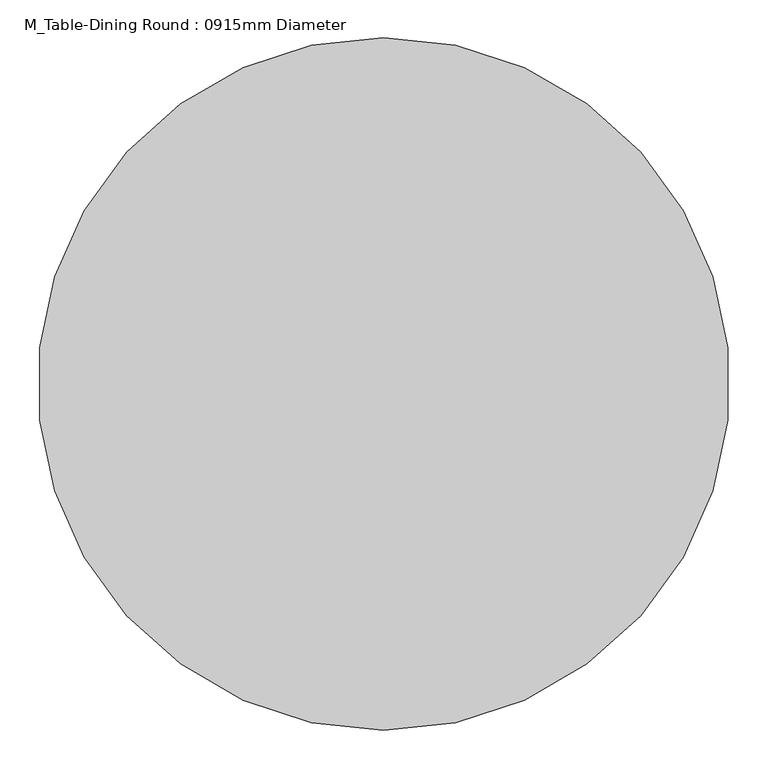
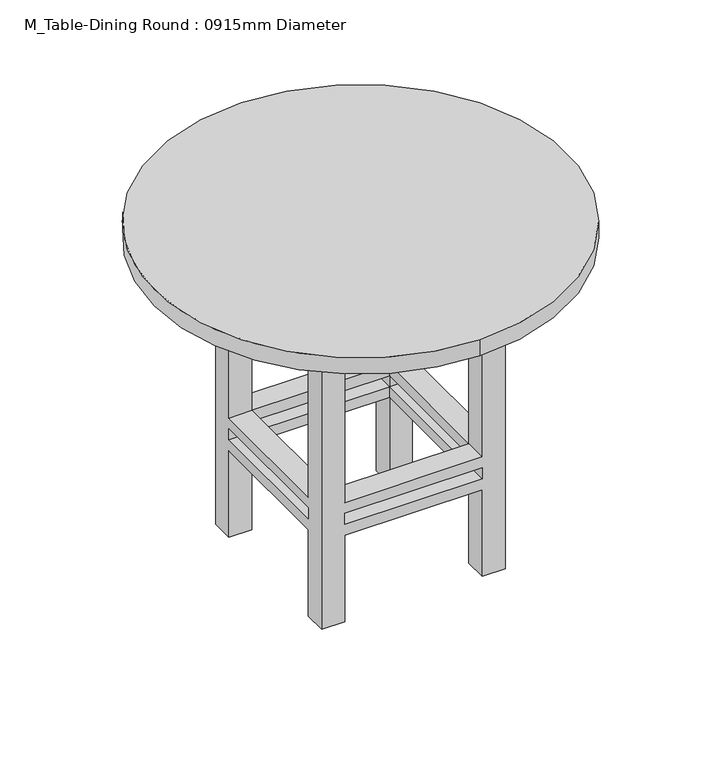
"""IFC4 building model written with IfcOpenShell, lengths in millimetres: furniture geometry, M_Table-Dining Round : 0915mm Diameter."""

from ifc_helpers import new_model, si_unit, point, frame, frame_2d, origin, place, context, project, spatial, polyline, circle_curve, trimmed, segment, composite_curve, outline, extrude, faceted_brep, source, transform, mapped, element, save


def m_table_dining_round_0915mm_diameter_394c0b6d(model_context):
    return source(origin(), model_context, "Body", "SolidModel", [
        extrude(outline(polyline([(332.4319672, 43.8713115), (332.4319672, -413.6286885), (-125.0680328, -413.6286885), (-125.0680328, 43.8713115), (332.4319672, 43.8713115)]), holes=[polyline([(307.0319672, 18.4713115), (-99.6680328, 18.4713115), (-99.6680328, -388.2286885), (307.0319672, -388.2286885), (307.0319672, 18.4713115)])]), frame((0.0, 0.0, 647.7), z_axis=(0.0, 0.0, 1.0), x_axis=(1.0, 0.0, 0.0)), (0.0, 0.0, 1.0), 76.2),
        faceted_brep([(-48.8680328, 18.4713115, 647.7), (-99.6680328, 18.4713115, 647.7), (-99.6680328, -32.3286885, 647.7), (-48.8680328, -32.3286885, 647.7), (256.2319672, 18.4713115, 647.7), (256.2319672, -32.3286885, 647.7), (307.0319672, -32.3286885, 647.7), (307.0319672, 18.4713115, 647.7), (256.2319672, -388.2286885, 647.7), (307.0319672, -388.2286885, 647.7), (307.0319672, -337.4286885, 647.7), (256.2319672, -337.4286885, 647.7), (-48.8680328, -388.2286885, 647.7), (-48.8680328, -337.4286885, 647.7), (-99.6680328, -337.4286885, 647.7), (-99.6680328, -388.2286885, 647.7), (-48.8680328, 18.4713115, 0.0), (-48.8680328, -32.3286885, 0.0), (-99.6680328, -32.3286885, 0.0), (-99.6680328, 18.4713115, 0.0), (256.2319672, 18.4713115, 0.0), (307.0319672, 18.4713115, 0.0), (307.0319672, -32.3286885, 0.0), (256.2319672, -32.3286885, 0.0), (256.2319672, -388.2286885, 0.0), (256.2319672, -337.4286885, 0.0), (307.0319672, -337.4286885, 0.0), (307.0319672, -388.2286885, 0.0), (-48.8680328, -388.2286885, 0.0), (-99.6680328, -388.2286885, 0.0), (-99.6680328, -337.4286885, 0.0), (-48.8680328, -337.4286885, 0.0), (-48.8680328, 18.4713115, 279.4), (256.2319672, 18.4713115, 279.4), (256.2319672, 18.4713115, 203.2), (-48.8680328, 18.4713115, 203.2), (256.2319672, 18.4713115, 228.6), (256.2319672, 18.4713115, 254.0), (-48.8680328, 18.4713115, 254.0), (-48.8680328, 18.4713115, 228.6), (-99.6680328, -32.3286885, 203.2), (-99.6680328, -337.4286885, 203.2), (-99.6680328, -337.4286885, 279.4), (-99.6680328, -32.3286885, 279.4), (-99.6680328, -32.3286885, 228.6), (-99.6680328, -32.3286885, 254.0), (-99.6680328, -337.4286885, 254.0), (-99.6680328, -337.4286885, 228.6), (-48.8680328, -32.3286885, 279.4), (-48.8680328, -32.3286885, 203.2), (-48.8680328, -32.3286885, 228.6), (-48.8680328, -32.3286885, 254.0), (256.2319672, -32.3286885, 279.4), (256.2319672, -32.3286885, 203.2), (256.2319672, -32.3286885, 228.6), (256.2319672, -32.3286885, 254.0), (307.0319672, -32.3286885, 279.4), (307.0319672, -32.3286885, 203.2), (307.0319672, -32.3286885, 228.6), (307.0319672, -32.3286885, 254.0), (307.0319672, -337.4286885, 279.4), (307.0319672, -337.4286885, 203.2), (307.0319672, -337.4286885, 228.6), (307.0319672, -337.4286885, 254.0), (256.2319672, -388.2286885, 279.4), (-48.8680328, -388.2286885, 279.4), (-48.8680328, -388.2286885, 203.2), (256.2319672, -388.2286885, 203.2), (-48.8680328, -388.2286885, 228.6), (-48.8680328, -388.2286885, 254.0), (256.2319672, -388.2286885, 254.0), (256.2319672, -388.2286885, 228.6), (256.2319672, -337.4286885, 279.4), (256.2319672, -337.4286885, 203.2), (256.2319672, -337.4286885, 228.6), (256.2319672, -337.4286885, 254.0), (-48.8680328, -337.4286885, 279.4), (-48.8680328, -337.4286885, 203.2), (-48.8680328, -337.4286885, 228.6), (-48.8680328, -337.4286885, 254.0)], [[[0, 1, 2, 3]], [[4, 5, 6, 7]], [[8, 9, 10, 11]], [[12, 13, 14, 15]], [[16, 17, 18, 19]], [[20, 21, 22, 23]], [[24, 25, 26, 27]], [[28, 29, 30, 31]], [[1, 0, 32, 33, 4, 7, 21, 20, 34, 35, 16, 19], [36, 37, 38, 39]], [[2, 1, 19, 18, 40, 41, 30, 29, 15, 14, 42, 43], [44, 45, 46, 47]], [[3, 2, 43, 48]], [[18, 17, 49, 40]], [[44, 50, 51, 45]], [[0, 3, 48, 32]], [[17, 16, 35, 49]], [[50, 39, 38, 51]], [[5, 4, 33, 52]], [[20, 23, 53, 34]], [[36, 54, 55, 37]], [[6, 5, 52, 56]], [[23, 22, 57, 53]], [[54, 58, 59, 55]], [[21, 7, 6, 56, 60, 10, 9, 27, 26, 61, 57, 22], [62, 63, 59, 58]], [[27, 9, 8, 64, 65, 12, 15, 29, 28, 66, 67, 24], [68, 69, 70, 71]], [[11, 10, 60, 72]], [[26, 25, 73, 61]], [[62, 74, 75, 63]], [[8, 11, 72, 64]], [[25, 24, 67, 73]], [[74, 71, 70, 75]], [[13, 12, 65, 76]], [[28, 31, 77, 66]], [[68, 78, 79, 69]], [[14, 13, 76, 42]], [[31, 30, 41, 77]], [[78, 47, 46, 79]], [[54, 74, 62, 58]], [[74, 78, 68, 71]], [[78, 50, 44, 47]], [[50, 54, 36, 39]], [[53, 49, 35, 34]], [[49, 77, 41, 40]], [[77, 73, 67, 66]], [[73, 53, 57, 61]], [[74, 54, 53, 73]], [[78, 74, 73, 77]], [[50, 78, 77, 49]], [[54, 50, 49, 53]], [[52, 72, 60, 56]], [[72, 76, 65, 64]], [[76, 48, 43, 42]], [[48, 52, 33, 32]], [[55, 51, 38, 37]], [[51, 79, 46, 45]], [[79, 75, 70, 69]], [[75, 55, 59, 63]], [[72, 52, 55, 75]], [[76, 72, 75, 79]], [[48, 76, 79, 51]], [[52, 48, 51, 55]]]),
        extrude(outline(composite_curve([segment(trimmed(circle_curve(frame_2d((103.6819672, -184.8786885)), 457.5), [point((103.6819672, -642.3786885))], [point((103.6819672, 272.6213115))], False, "CARTESIAN"), True, "CONTINUOUS"), segment(trimmed(circle_curve(frame_2d((103.6819672, -184.8786885)), 457.5), [point((103.6819672, 272.6213115))], [point((103.6819672, -642.3786885))], False, "CARTESIAN"), True, "CONTINUOUS")], self_intersect=False)), frame((0.0, 0.0, 723.9), z_axis=(0.0, 0.0, 1.0), x_axis=(1.0, 0.0, 0.0)), (0.0, 0.0, 1.0), 38.1),
    ])


if __name__ == "__main__":
    model = new_model("IFC4")
    model_context = context("Model", 3, world=origin())
    ifc_project = project(units=[si_unit("LENGTHUNIT", "METRE", prefix="MILLI")], contexts=[model_context])
    site = spatial("IfcSite", under=ifc_project)
    building = spatial("IfcBuilding", under=site)
    placement = place(None, origin())
    m_table_dining_round_0915mm_diameter_shape = m_table_dining_round_0915mm_diameter_394c0b6d(model_context)
    element("IfcFurniture", 1, ObjectType="M_Table-Dining Round : 0915mm Diameter", at=placement, inside=building, context=model_context, shape_type="MappedRepresentation", body=[
        mapped(m_table_dining_round_0915mm_diameter_shape, transform((0.0, 0.0, 0.0), x_axis=(1.0, 0.0, 0.0), y_axis=(0.0, 1.0, 0.0), z_axis=(0.0, 0.0, 1.0))),
    ])
    save(model, "model.ifc")

# Revit data of these elements
# Type "M_Table-Dining Round : 0915mm Diameter"
#   Diameter = 3.001969 ft
#   Height = 2.5 ft
#   Base Material = Pine
#   Top Material = Laminate, Linen, Matte
#   Default Elevation = 0
# Element 1 (IfcFurniture, "M_Table-Dining Round : 0915mm Diameter")
#   Materials on its faces: "Pine", "Laminate, Linen, Matte"
# Materials
#   "Pine": class "Wood", colour RGB 223 192 134, transparency 0, Description = "Pinus Echinata", Cost = 0
#   "Laminate, Linen, Matte": class "Plastic", colour RGB 249 239 230, transparency 0, Description = "Plastic Laminate - Linen, Matte", Cost = 0
